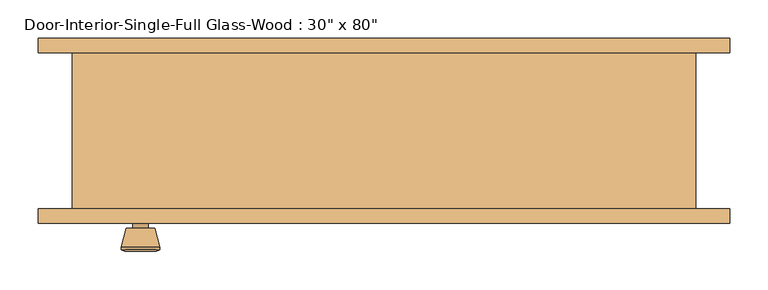
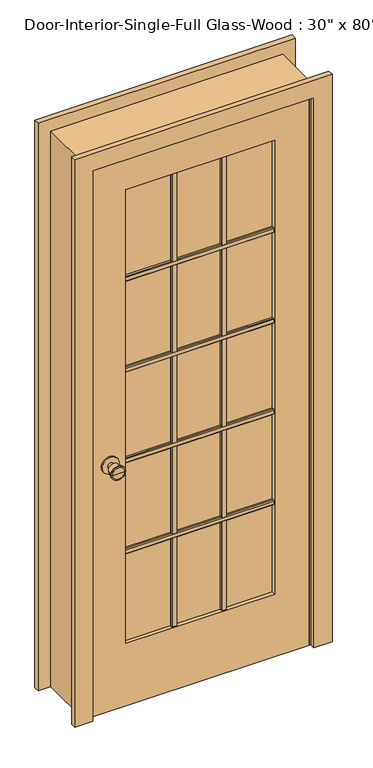
"""IFC4 building model written with IfcOpenShell, lengths in millimetres: door geometry."""

from ifc_helpers import new_model, si_unit, point, frame, frame_2d, origin, place, context, project, spatial, polyline, circle_curve, trimmed, segment, composite_curve, outline, extrude, faceted_brep, source, transform, mapped, element, save
from ifc_brep_helpers import plane_surface, cylinder_surface, revolved_surface, advanced_brep


def door_d788789e(model_context):
    return source(origin(), model_context, "Body", "SolidModel", [
        extrude(outline(polyline([(-84.455, 1586.23), (-84.455, 1567.18), (-90.805, 1567.18), (-93.98, 1570.355), (-93.98, 1583.055), (-90.805, 1586.23), (-84.455, 1586.23)])), frame((-260.35, 0.0, 0.0), z_axis=(1.0, 0.0, 0.0), x_axis=(0.0, 1.0, 0.0)), (0.0, 0.0, 1.0), 520.7),
        extrude(outline(polyline([(-84.455, 1249.9975), (-84.455, 1230.9475), (-90.805, 1230.9475), (-93.98, 1234.1225), (-93.98, 1246.8225), (-90.805, 1249.9975), (-84.455, 1249.9975)])), frame((-260.35, 0.0, 0.0), z_axis=(1.0, 0.0, 0.0), x_axis=(0.0, 1.0, 0.0)), (0.0, 0.0, 1.0), 520.7),
        extrude(outline(polyline([(-84.455, 913.765), (-84.455, 894.715), (-90.805, 894.715), (-93.98, 897.89), (-93.98, 910.59), (-90.805, 913.765), (-84.455, 913.765)])), frame((-260.35, 0.0, 0.0), z_axis=(1.0, 0.0, 0.0), x_axis=(0.0, 1.0, 0.0)), (0.0, 0.0, 1.0), 520.7),
        extrude(outline(polyline([(-84.455, 577.5325), (-84.455, 558.4825), (-90.805, 558.4825), (-93.98, 561.6575), (-93.98, 574.3575), (-90.805, 577.5325), (-84.455, 577.5325)])), frame((-260.35, 0.0, 0.0), z_axis=(1.0, 0.0, 0.0), x_axis=(0.0, 1.0, 0.0)), (0.0, 0.0, 1.0), 520.7),
        extrude(outline(polyline([(77.2583333, -84.455), (96.3083333, -84.455), (96.3083333, -90.805), (93.1333333, -93.98), (80.4333333, -93.98), (77.2583333, -90.805), (77.2583333, -84.455)])), frame((0.0, 0.0, 231.775), z_axis=(0.0, 0.0, 1.0), x_axis=(1.0, 0.0, 0.0)), (0.0, 0.0, 1.0), 1681.1625),
        extrude(outline(polyline([(-96.3083333, -84.455), (-77.2583333, -84.455), (-77.2583333, -90.805), (-80.4333333, -93.98), (-93.1333333, -93.98), (-96.3083333, -90.805), (-96.3083333, -84.455)])), frame((0.0, 0.0, 231.775), z_axis=(0.0, 0.0, 1.0), x_axis=(1.0, 0.0, 0.0)), (0.0, 0.0, 1.0), 1681.1625),
        extrude(outline(polyline([(-77.47, 1586.23), (-71.12, 1586.23), (-67.945, 1583.055), (-67.945, 1570.355), (-71.12, 1567.18), (-77.47, 1567.18), (-77.47, 1586.23)])), frame((-260.35, 0.0, 0.0), z_axis=(1.0, 0.0, 0.0), x_axis=(0.0, 1.0, 0.0)), (0.0, 0.0, 1.0), 520.7),
        extrude(outline(polyline([(-77.47, 1249.9975), (-71.12, 1249.9975), (-67.945, 1246.8225), (-67.945, 1234.1225), (-71.12, 1230.9475), (-77.47, 1230.9475), (-77.47, 1249.9975)])), frame((-260.35, 0.0, 0.0), z_axis=(1.0, 0.0, 0.0), x_axis=(0.0, 1.0, 0.0)), (0.0, 0.0, 1.0), 520.7),
        extrude(outline(polyline([(-77.47, 913.765), (-71.12, 913.765), (-67.945, 910.59), (-67.945, 897.89), (-71.12, 894.715), (-77.47, 894.715), (-77.47, 913.765)])), frame((-260.35, 0.0, 0.0), z_axis=(1.0, 0.0, 0.0), x_axis=(0.0, 1.0, 0.0)), (0.0, 0.0, 1.0), 520.7),
        extrude(outline(polyline([(-77.47, 577.5325), (-71.12, 577.5325), (-67.945, 574.3575), (-67.945, 561.6575), (-71.12, 558.4825), (-77.47, 558.4825), (-77.47, 577.5325)])), frame((-260.35, 0.0, 0.0), z_axis=(1.0, 0.0, 0.0), x_axis=(0.0, 1.0, 0.0)), (0.0, 0.0, 1.0), 520.7),
        extrude(outline(polyline([(77.2583333, -77.47), (77.2583333, -71.12), (80.4333333, -67.945), (93.1333333, -67.945), (96.3083333, -71.12), (96.3083333, -77.47), (77.2583333, -77.47)])), frame((0.0, 0.0, 231.775), z_axis=(0.0, 0.0, 1.0), x_axis=(1.0, 0.0, 0.0)), (0.0, 0.0, 1.0), 1681.1625),
        extrude(outline(polyline([(-96.3083333, -77.47), (-96.3083333, -71.12), (-93.1333333, -67.945), (-80.4333333, -67.945), (-77.2583333, -71.12), (-77.2583333, -77.47), (-96.3083333, -77.47)])), frame((0.0, 0.0, 231.775), z_axis=(0.0, 0.0, 1.0), x_axis=(1.0, 0.0, 0.0)), (0.0, 0.0, 1.0), 1681.1625),
        advanced_brep(
        [(-317.5, -57.5, 914.4), (-327.5, -57.5, 914.4), (-307.5, -57.5, 914.4), (-297.0241324, -8.5, 914.4), (-337.9758676, -8.5, 914.4), (-317.5, -8.5, 914.4), (-292.5, -10.3278681, 914.4), (-342.5, -10.3278681, 914.4), (-292.5, -13.7915463, 914.4), (-342.5, -13.7915463, 914.4), (-298.863764, -38.5, 914.4), (-336.136236, -38.5, 914.4), (-307.5, -38.5, 914.4), (-327.5, -38.5, 914.4)],
        [
            (0, 1),
            (1, 2, circle_curve(frame((-317.5, -57.5, 914.4), z_axis=(0.0, -1.0, 0.0), x_axis=(-1.0, 0.0, 0.0)), 10.0)),
            (2, 0),
            (2, 1, circle_curve(frame((-317.5, -57.5, 914.4), z_axis=(0.0, -1.0, 0.0), x_axis=(-1.0, 0.0, 0.0)), 10.0)),
            (3, 4, circle_curve(frame((-317.5, -8.5, 914.4), z_axis=(0.0, 1.0, 0.0), x_axis=(-1.0, 0.0, 0.0)), 20.4758676)),
            (4, 5),
            (5, 3),
            (4, 3, circle_curve(frame((-317.5, -8.5, 914.4), z_axis=(0.0, 1.0, 0.0), x_axis=(-1.0, 0.0, 0.0)), 20.4758676)),
            (6, 7, circle_curve(frame((-317.5, -10.3278681, 914.4), z_axis=(0.0, 1.0, 0.0), x_axis=(-1.0, 0.0, 0.0)), 25.0)),
            (7, 4),
            (3, 6),
            (7, 6, circle_curve(frame((-317.5, -10.3278681, 914.4), z_axis=(0.0, 1.0, 0.0), x_axis=(-1.0, 0.0, 0.0)), 25.0)),
            (8, 9, circle_curve(frame((-317.5, -13.7915463, 914.4), z_axis=(0.0, 1.0, 0.0), x_axis=(-1.0, 0.0, 0.0)), 25.0)),
            (9, 7),
            (6, 8),
            (9, 8, circle_curve(frame((-317.5, -13.7915463, 914.4), z_axis=(0.0, 1.0, 0.0), x_axis=(-1.0, 0.0, 0.0)), 25.0)),
            (10, 11, circle_curve(frame((-317.5, -38.5, 914.4), z_axis=(0.0, 1.0, 0.0), x_axis=(-1.0, 0.0, 0.0)), 18.636236)),
            (11, 9),
            (8, 10),
            (11, 10, circle_curve(frame((-317.5, -38.5, 914.4), z_axis=(0.0, 1.0, 0.0), x_axis=(-1.0, 0.0, 0.0)), 18.636236)),
            (12, 13, circle_curve(frame((-317.5, -38.5, 914.4), z_axis=(0.0, 1.0, 0.0), x_axis=(-1.0, 0.0, 0.0)), 10.0)),
            (13, 11),
            (10, 12),
            (13, 12, circle_curve(frame((-317.5, -38.5, 914.4), z_axis=(0.0, 1.0, 0.0), x_axis=(-1.0, 0.0, 0.0)), 10.0)),
            (1, 13),
            (12, 2),
        ],
        [
            plane_surface(frame((-317.5, -57.5, 914.4), z_axis=(0.0, -1.0, 0.0), x_axis=(-1.0, 0.0, 0.0))),
            plane_surface(frame((-317.5, -8.5, 914.4), z_axis=(0.0, 1.0, 0.0), x_axis=(-1.0, 0.0, 0.0))),
            revolved_surface(polyline([(-337.9758676, -8.5, 914.4), (-342.5, -10.3278681, 914.4)]), (-317.5, -57.5, 914.4), (0.0, -1.0, 0.0)),
            cylinder_surface(frame((-317.5, -57.5, 914.4), z_axis=(0.0, -1.0, 0.0), x_axis=(-1.0, 0.0, 0.0)), 25.0),
            revolved_surface(polyline([(-342.5, -13.7915463, 914.4), (-336.136236, -38.5, 914.4)]), (-317.5, -57.5, 914.4), (0.0, -1.0, 0.0)),
            plane_surface(frame((-317.5, -38.5, 914.4), z_axis=(0.0, -1.0, 0.0), x_axis=(-1.0, 0.0, 0.0))),
            cylinder_surface(frame((-317.5, -57.5, 914.4), z_axis=(0.0, -1.0, 0.0), x_axis=(-1.0, 0.0, 0.0)), 10.0),
        ],
        [
            (0, [[1, 2, 3]]),
            (0, [[-3, 4, -1]]),
            (1, [[5, 6, 7]]),
            (1, [[8, -7, -6]]),
            (2, [[9, 10, -5, 11]]),
            (2, [[12, -11, -8, -10]]),
            (3, [[13, 14, -9, 15]]),
            (3, [[16, -15, -12, -14]]),
            (4, [[17, 18, -13, 19]]),
            (4, [[20, -19, -16, -18]]),
            (5, [[21, 22, -17, 23]]),
            (5, [[24, -23, -20, -22]]),
            (6, [[-2, 25, -21, 26]]),
            (6, [[-4, -26, -24, -25]]),
        ],
    ),
        extrude(outline(composite_curve([segment(trimmed(circle_curve(frame_2d((914.4, -317.5)), 30.0), [point((914.4, -347.5))], [point((914.4, -287.5))], False, "CARTESIAN"), True, "CONTINUOUS"), segment(trimmed(circle_curve(frame_2d((914.4, -317.5)), 30.0), [point((914.4, -287.5))], [point((914.4, -347.5))], False, "CARTESIAN"), True, "CONTINUOUS")], self_intersect=False)), frame((0.0, -63.5, 0.0), z_axis=(0.0, 1.0, 0.0), x_axis=(0.0, 0.0, 1.0)), (0.0, 0.0, 1.0), 6.0),
        advanced_brep(
        [(-317.5, -104.425, 914.4), (-307.5, -104.425, 914.4), (-327.5, -104.425, 914.4), (-297.0241324, -153.425, 914.4), (-317.5, -153.425, 914.4), (-337.9758676, -153.425, 914.4), (-292.5, -151.5971319, 914.4), (-342.5, -151.5971319, 914.4), (-292.5, -148.1334537, 914.4), (-342.5, -148.1334537, 914.4), (-298.863764, -123.425, 914.4), (-336.136236, -123.425, 914.4), (-307.5, -123.425, 914.4), (-327.5, -123.425, 914.4)],
        [
            (0, 1),
            (1, 2, circle_curve(frame((-317.5, -104.425, 914.4), z_axis=(0.0, 1.0, 0.0), x_axis=(-1.0, 0.0, 0.0)), 10.0)),
            (2, 0),
            (2, 1, circle_curve(frame((-317.5, -104.425, 914.4), z_axis=(0.0, 1.0, 0.0), x_axis=(-1.0, 0.0, 0.0)), 10.0)),
            (3, 4),
            (4, 5),
            (5, 3, circle_curve(frame((-317.5, -153.425, 914.4), z_axis=(0.0, -1.0, 0.0), x_axis=(-1.0, 0.0, 0.0)), 20.4758676)),
            (3, 5, circle_curve(frame((-317.5, -153.425, 914.4), z_axis=(0.0, -1.0, 0.0), x_axis=(-1.0, 0.0, 0.0)), 20.4758676)),
            (6, 3),
            (5, 7),
            (7, 6, circle_curve(frame((-317.5, -151.5971319, 914.4), z_axis=(0.0, -1.0, 0.0), x_axis=(-1.0, 0.0, 0.0)), 25.0)),
            (6, 7, circle_curve(frame((-317.5, -151.5971319, 914.4), z_axis=(0.0, -1.0, 0.0), x_axis=(-1.0, 0.0, 0.0)), 25.0)),
            (8, 6),
            (7, 9),
            (9, 8, circle_curve(frame((-317.5, -148.1334537, 914.4), z_axis=(0.0, -1.0, 0.0), x_axis=(-1.0, 0.0, 0.0)), 25.0)),
            (8, 9, circle_curve(frame((-317.5, -148.1334537, 914.4), z_axis=(0.0, -1.0, 0.0), x_axis=(-1.0, 0.0, 0.0)), 25.0)),
            (10, 8),
            (9, 11),
            (11, 10, circle_curve(frame((-317.5, -123.425, 914.4), z_axis=(0.0, -1.0, 0.0), x_axis=(-1.0, 0.0, 0.0)), 18.636236)),
            (10, 11, circle_curve(frame((-317.5, -123.425, 914.4), z_axis=(0.0, -1.0, 0.0), x_axis=(-1.0, 0.0, 0.0)), 18.636236)),
            (12, 10),
            (11, 13),
            (13, 12, circle_curve(frame((-317.5, -123.425, 914.4), z_axis=(0.0, -1.0, 0.0), x_axis=(-1.0, 0.0, 0.0)), 10.0)),
            (12, 13, circle_curve(frame((-317.5, -123.425, 914.4), z_axis=(0.0, -1.0, 0.0), x_axis=(-1.0, 0.0, 0.0)), 10.0)),
            (1, 12),
            (13, 2),
        ],
        [
            plane_surface(frame((-317.5, -104.425, 914.4), z_axis=(0.0, 1.0, 0.0), x_axis=(-1.0, 0.0, 0.0))),
            plane_surface(frame((-317.5, -153.425, 914.4), z_axis=(0.0, -1.0, 0.0), x_axis=(-1.0, 0.0, 0.0))),
            revolved_surface(polyline([(-337.9758676, -153.425, 914.4), (-342.5, -151.5971319, 914.4)]), (-317.5, -104.425, 914.4), (0.0, 1.0, 0.0)),
            cylinder_surface(frame((-317.5, -104.425, 914.4), z_axis=(0.0, 1.0, 0.0), x_axis=(-1.0, 0.0, 0.0)), 25.0),
            revolved_surface(polyline([(-342.5, -148.1334537, 914.4), (-336.136236, -123.425, 914.4)]), (-317.5, -104.425, 914.4), (0.0, 1.0, 0.0)),
            plane_surface(frame((-317.5, -123.425, 914.4), z_axis=(0.0, 1.0, 0.0), x_axis=(-1.0, 0.0, 0.0))),
            cylinder_surface(frame((-317.5, -104.425, 914.4), z_axis=(0.0, 1.0, 0.0), x_axis=(-1.0, 0.0, 0.0)), 10.0),
        ],
        [
            (0, [[1, 2, 3]]),
            (0, [[-3, 4, -1]]),
            (1, [[5, 6, 7]]),
            (1, [[-6, -5, 8]]),
            (2, [[9, -7, 10, 11]]),
            (2, [[-10, -8, -9, 12]]),
            (3, [[13, -11, 14, 15]]),
            (3, [[-14, -12, -13, 16]]),
            (4, [[17, -15, 18, 19]]),
            (4, [[-18, -16, -17, 20]]),
            (5, [[21, -19, 22, 23]]),
            (5, [[-22, -20, -21, 24]]),
            (6, [[25, -23, 26, -2]]),
            (6, [[-26, -24, -25, -4]]),
        ],
    ),
        extrude(outline(composite_curve([segment(trimmed(circle_curve(frame_2d((914.4, -317.5)), 30.0), [point((914.4, -347.5))], [point((914.4, -287.5))], False, "CARTESIAN"), True, "CONTINUOUS"), segment(trimmed(circle_curve(frame_2d((914.4, -317.5)), 30.0), [point((914.4, -287.5))], [point((914.4, -347.5))], False, "CARTESIAN"), True, "CONTINUOUS")], self_intersect=False)), frame((0.0, -104.425, 0.0), z_axis=(0.0, 1.0, 0.0), x_axis=(0.0, 0.0, 1.0)), (0.0, 0.0, 1.0), 6.0),
        extrude(outline(polyline([(2032.0, -381.0), (0.0, -381.0), (0.0, 381.0), (2032.0, 381.0), (2032.0, -381.0)]), holes=[polyline([(1912.9375, -260.35), (1912.9375, 260.35), (231.775, 260.35), (231.775, -260.35), (1912.9375, -260.35)])]), frame((0.0, -98.425, 0.0), z_axis=(0.0, 1.0, 0.0), x_axis=(0.0, 0.0, 1.0)), (0.0, 0.0, 1.0), 34.925),
        faceted_brep([(406.4, -98.425, 0.0), (381.0, -98.425, 0.0), (381.0, -63.5, 0.0), (368.3, -63.5, 0.0), (368.3, -28.575, 0.0), (381.0, -28.575, 0.0), (381.0, 104.775, 0.0), (406.4, 104.775, 0.0), (406.4, 104.775, 2057.4), (406.4, -98.425, 2057.4), (381.0, 104.775, 2032.0), (-381.0, 104.775, 2032.0), (-381.0, 104.775, 0.0), (-406.4, 104.775, 0.0), (-406.4, 104.775, 2057.4), (381.0, -28.575, 2032.0), (368.3, -28.575, 2019.3), (-368.3, -28.575, 2019.3), (-368.3, -28.575, 0.0), (-381.0, -28.575, 0.0), (-381.0, -28.575, 2032.0), (368.3, -63.5, 2019.3), (381.0, -63.5, 2032.0), (-381.0, -63.5, 2032.0), (-381.0, -63.5, 0.0), (-368.3, -63.5, 0.0), (-368.3, -63.5, 2019.3), (381.0, -98.425, 2032.0), (-406.4, -98.425, 2057.4), (-406.4, -98.425, 0.0), (-381.0, -98.425, 0.0), (-381.0, -98.425, 2032.0)], [[[0, 1, 2, 3, 4, 5, 6, 7]], [[7, 8, 9, 0]], [[6, 10, 11, 12, 13, 14, 8, 7]], [[5, 15, 10, 6]], [[4, 16, 17, 18, 19, 20, 15, 5]], [[3, 21, 16, 4]], [[2, 22, 23, 24, 25, 26, 21, 3]], [[1, 27, 22, 2]], [[0, 9, 28, 29, 30, 31, 27, 1]], [[8, 14, 28, 9]], [[15, 20, 11, 10]], [[21, 26, 17, 16]], [[27, 31, 23, 22]], [[29, 13, 12, 19, 18, 25, 24, 30]], [[14, 13, 29, 28]], [[20, 19, 12, 11]], [[26, 25, 18, 17]], [[31, 30, 24, 23]]]),
        extrude(outline(polyline([(260.35, -77.47), (260.35, -84.455), (-260.35, -84.455), (-260.35, -77.47), (260.35, -77.47)])), frame((0.0, 0.0, 231.775), z_axis=(0.0, 0.0, 1.0), x_axis=(1.0, 0.0, 0.0)), (0.0, 0.0, 1.0), 1681.1625),
        extrude(outline(polyline([(0.0, 450.85), (2101.85, 450.85), (2101.85, -450.85), (0.0, -450.85), (0.0, -387.35), (2038.35, -387.35), (2038.35, 387.35), (0.0, 387.35), (0.0, 450.85)])), frame((0.0, 104.775, 0.0), z_axis=(0.0, 1.0, 0.0), x_axis=(0.0, 0.0, 1.0)), (0.0, 0.0, 1.0), 19.05),
        extrude(outline(polyline([(0.0, 450.85), (2101.85, 450.85), (2101.85, -450.85), (0.0, -450.85), (0.0, -387.35), (2038.35, -387.35), (2038.35, 387.35), (0.0, 387.35), (0.0, 450.85)])), frame((0.0, -117.475, 0.0), z_axis=(0.0, 1.0, 0.0), x_axis=(0.0, 0.0, 1.0)), (0.0, 0.0, 1.0), 19.05),
    ])


if __name__ == "__main__":
    model = new_model("IFC4")
    model_context = context("Model", 3, world=origin())
    ifc_project = project(units=[si_unit("LENGTHUNIT", "METRE", prefix="MILLI")], contexts=[model_context])
    site = spatial("IfcSite", under=ifc_project)
    building = spatial("IfcBuilding", under=site)
    placement = place(None, origin())
    door_shape = door_d788789e(model_context)
    element("IfcDoor", 1, ObjectType="Door-Interior-Single-Full Glass-Wood : 30\" x 80\"", at=placement, inside=building, context=model_context, shape_type="MappedRepresentation", body=[
        mapped(door_shape, transform((0.0, 0.0, 0.0), x_axis=(1.0, 0.0, 0.0), y_axis=(0.0, 1.0, 0.0), z_axis=(0.0, 0.0, 1.0))),
    ])
    save(model, "model.ifc")

# Revit data of these elements
# Type "Door-Interior-Single-Full Glass-Wood : 30\" x 80\""
#   Type Mark = "10"
#   Assembly Code = "C1020300"
#   Analytic Construction = "Wood frame with single clear glass"
#   Top Rail = 0' - 4 11/16"
#   Thickness = 0' - 1 3/8"
#   Thermal Resistance (R) = 1.0102 (h·ft²·°F)/BTU
#   Swing Angle [instance default] = 90.00°
#   Stiles = 0' - 4 3/4"
#   Rough Width = 2' - 8"
#   Rough Height = 6' - 9"
#   Height = 6' - 8"
#   Width = 2' - 6"
#   Heat Transfer Coefficient (U) = 0.9900 BTU/(h·ft²·°F)
#   Bottom Rail = 0' - 9 1/8"
#   Show Grill [instance default] = yes
#   Trim Material = Cherry
#   Panel Material = Cherry
#   Frame Material = Cherry
#   Door Handle Material = Aluminum
#   Visual Light Transmittance = 0
#   Solar Heat Gain Coefficient = 0
#   Wall Closure = (empty or 0)
#   Function = (empty or 0)
# Element 1 (IfcDoor, "Door-Interior-Single-Full Glass-Wood : 30\" x 80\"")
#   Materials on its faces: "Cherry", "Aluminum", "Glass"
# Materials
#   "Cherry": class "Wood", colour RGB 226 177 128, transparency 0, Description = "Prunus Serotina", Cost = 0
#   "Aluminum": class "Metal", colour RGB 247 247 247, transparency 0, Description = "Aluminum 6061", Cost = 0
#   "Glass": class "Glass", colour RGB 0 128 192, transparency 0.75, Description = "Soda Lime Glass", Cost = 0
